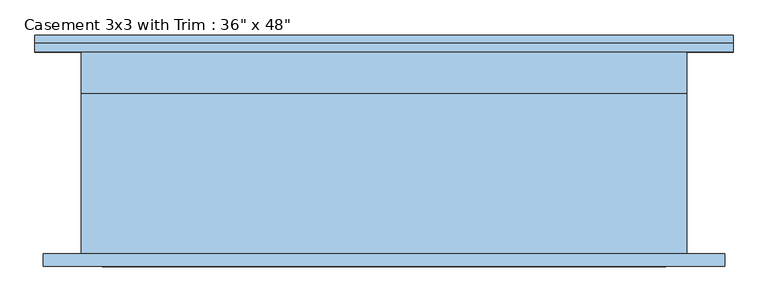
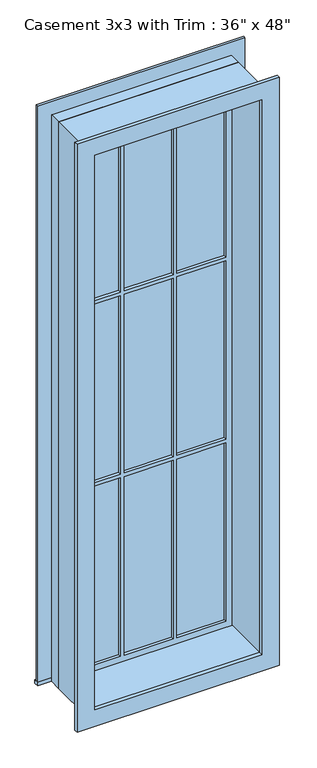
"""IFC4 building model written with IfcOpenShell, lengths in millimetres: window geometry."""

from ifc_helpers import new_model, si_unit, frame, origin, place, context, project, spatial, polyline, outline, extrude, source, transform, mapped, element, save


def window_19f256ab(model_context):
    return source(origin(), model_context, "Body", "SweptSolid", [
        extrude(outline(polyline([(-527.05, 177.8), (527.05, 177.8), (527.05, 152.4), (-527.05, 152.4), (-527.05, 177.8)])), frame((0.0, 0.0, 914.4), z_axis=(0.0, 0.0, 1.0), x_axis=(1.0, 0.0, 0.0)), (0.0, 0.0, 1.0), 19.05),
        extrude(outline(polyline([(3943.35, -438.15), (3943.35, 438.15), (933.45, 438.15), (933.45, 527.05), (4032.25, 527.05), (4032.25, -527.05), (933.45, -527.05), (933.45, -438.15), (3943.35, -438.15)])), frame((0.0, 152.4, 0.0), z_axis=(0.0, 1.0, 0.0), x_axis=(0.0, 0.0, 1.0)), (0.0, 0.0, 1.0), 12.7),
        extrude(outline(polyline([(143.9333333, 117.475), (393.7, 117.475), (393.7, 104.775), (143.9333333, 104.775), (143.9333333, 117.475)])), frame((0.0, 0.0, 2937.9333333), z_axis=(0.0, 0.0, 1.0), x_axis=(1.0, 0.0, 0.0)), (0.0, 0.0, 1.0), 960.9666667),
        extrude(outline(polyline([(-124.8833333, 117.475), (124.8833333, 117.475), (124.8833333, 104.775), (-124.8833333, 104.775), (-124.8833333, 117.475)])), frame((0.0, 0.0, 2937.9333333), z_axis=(0.0, 0.0, 1.0), x_axis=(1.0, 0.0, 0.0)), (0.0, 0.0, 1.0), 960.9666667),
        extrude(outline(polyline([(-393.7, 117.475), (-143.9333333, 117.475), (-143.9333333, 104.775), (-393.7, 104.775), (-393.7, 117.475)])), frame((0.0, 0.0, 2937.9333333), z_axis=(0.0, 0.0, 1.0), x_axis=(1.0, 0.0, 0.0)), (0.0, 0.0, 1.0), 960.9666667),
        extrude(outline(polyline([(-393.7, 117.475), (-143.9333333, 117.475), (-143.9333333, 104.775), (-393.7, 104.775), (-393.7, 117.475)])), frame((0.0, 0.0, 1957.9166667), z_axis=(0.0, 0.0, 1.0), x_axis=(1.0, 0.0, 0.0)), (0.0, 0.0, 1.0), 960.9666667),
        extrude(outline(polyline([(-124.8833333, 117.475), (124.8833333, 117.475), (124.8833333, 104.775), (-124.8833333, 104.775), (-124.8833333, 117.475)])), frame((0.0, 0.0, 1957.9166667), z_axis=(0.0, 0.0, 1.0), x_axis=(1.0, 0.0, 0.0)), (0.0, 0.0, 1.0), 960.9666667),
        extrude(outline(polyline([(143.9333333, 117.475), (393.7, 117.475), (393.7, 104.775), (143.9333333, 104.775), (143.9333333, 117.475)])), frame((0.0, 0.0, 1957.9166667), z_axis=(0.0, 0.0, 1.0), x_axis=(1.0, 0.0, 0.0)), (0.0, 0.0, 1.0), 960.9666667),
        extrude(outline(polyline([(143.9333333, 117.475), (393.7, 117.475), (393.7, 104.775), (143.9333333, 104.775), (143.9333333, 117.475)])), frame((0.0, 0.0, 977.9), z_axis=(0.0, 0.0, 1.0), x_axis=(1.0, 0.0, 0.0)), (0.0, 0.0, 1.0), 960.9666667),
        extrude(outline(polyline([(-124.8833333, 117.475), (124.8833333, 117.475), (124.8833333, 104.775), (-124.8833333, 104.775), (-124.8833333, 117.475)])), frame((0.0, 0.0, 977.9), z_axis=(0.0, 0.0, 1.0), x_axis=(1.0, 0.0, 0.0)), (0.0, 0.0, 1.0), 960.9666667),
        extrude(outline(polyline([(-393.7, 117.475), (-143.9333333, 117.475), (-143.9333333, 104.775), (-393.7, 104.775), (-393.7, 117.475)])), frame((0.0, 0.0, 977.9), z_axis=(0.0, 0.0, 1.0), x_axis=(1.0, 0.0, 0.0)), (0.0, 0.0, 1.0), 960.9666667),
        extrude(outline(polyline([(4019.55, 514.35), (4019.55, -514.35), (857.25, -514.35), (857.25, 514.35), (4019.55, 514.35)]), holes=[polyline([(3930.65, 425.45), (946.15, 425.45), (946.15, -425.45), (3930.65, -425.45), (3930.65, 425.45)])]), frame((0.0, -171.45, 0.0), z_axis=(0.0, 1.0, 0.0), x_axis=(0.0, 0.0, 1.0)), (0.0, 0.0, 1.0), 19.05),
        extrude(outline(polyline([(3943.35, -438.15), (933.45, -438.15), (933.45, 438.15), (3943.35, 438.15), (3943.35, -438.15)]), holes=[polyline([(3898.9, -143.9333333), (2937.9333333, -143.9333333), (2937.9333333, -393.7), (3898.9, -393.7), (3898.9, -143.9333333)]), polyline([(2918.8833333, -143.9333333), (1957.9166667, -143.9333333), (1957.9166667, -393.7), (2918.8833333, -393.7), (2918.8833333, -143.9333333)]), polyline([(1938.8666667, -143.9333333), (977.9, -143.9333333), (977.9, -393.7), (1938.8666667, -393.7), (1938.8666667, -143.9333333)]), polyline([(3898.9, 124.8833333), (2937.9333333, 124.8833333), (2937.9333333, -124.8833333), (3898.9, -124.8833333), (3898.9, 124.8833333)]), polyline([(2918.8833333, 124.8833333), (1957.9166667, 124.8833333), (1957.9166667, -124.8833333), (2918.8833333, -124.8833333), (2918.8833333, 124.8833333)]), polyline([(1938.8666667, 124.8833333), (977.9, 124.8833333), (977.9, -124.8833333), (1938.8666667, -124.8833333), (1938.8666667, 124.8833333)]), polyline([(3898.9, 393.7), (2937.9333333, 393.7), (2937.9333333, 143.9333333), (3898.9, 143.9333333), (3898.9, 393.7)]), polyline([(2918.8833333, 393.7), (1957.9166667, 393.7), (1957.9166667, 143.9333333), (2918.8833333, 143.9333333), (2918.8833333, 393.7)]), polyline([(1938.8666667, 393.7), (977.9, 393.7), (977.9, 143.9333333), (1938.8666667, 143.9333333), (1938.8666667, 393.7)])]), frame((0.0, 88.9, 0.0), z_axis=(0.0, 1.0, 0.0), x_axis=(0.0, 0.0, 1.0)), (0.0, 0.0, 1.0), 44.45),
        extrude(outline(polyline([(3962.4, -457.2), (914.4, -457.2), (914.4, 457.2), (3962.4, 457.2), (3962.4, -457.2)]), holes=[polyline([(3930.65, -425.45), (3930.65, 425.45), (946.15, 425.45), (946.15, -425.45), (3930.65, -425.45)])]), frame((0.0, -152.4, 0.0), z_axis=(0.0, 1.0, 0.0), x_axis=(0.0, 0.0, 1.0)), (0.0, 0.0, 1.0), 241.3),
        extrude(outline(polyline([(3962.4, 457.2), (3962.4, -457.2), (914.4, -457.2), (914.4, 457.2), (3962.4, 457.2)]), holes=[polyline([(3943.35, 438.15), (933.45, 438.15), (933.45, -438.15), (3943.35, -438.15), (3943.35, 438.15)])]), frame((0.0, 88.9, 0.0), z_axis=(0.0, 1.0, 0.0), x_axis=(0.0, 0.0, 1.0)), (0.0, 0.0, 1.0), 63.5),
    ])


if __name__ == "__main__":
    model = new_model("IFC4")
    model_context = context("Model", 3, world=origin())
    ifc_project = project(units=[si_unit("LENGTHUNIT", "METRE", prefix="MILLI")], contexts=[model_context])
    site = spatial("IfcSite", under=ifc_project)
    building = spatial("IfcBuilding", under=site)
    placement = place(None, origin())
    window_shape = window_19f256ab(model_context)
    element("IfcWindow", 1, ObjectType="Casement 3x3 with Trim : 36\" x 48\"", at=placement, inside=building, context=model_context, shape_type="MappedRepresentation", body=[
        mapped(window_shape, transform((0.0, 0.0, 0.0), x_axis=(1.0, 0.0, 0.0), y_axis=(0.0, 1.0, 0.0), z_axis=(0.0, 0.0, 1.0))),
    ])
    save(model, "model.ifc")

# Revit data of these elements
# Type "Casement 3x3 with Trim : 36\" x 48\""
#   Type Mark = "13"
#   Construction Type Id = "GSP4R"
#   Assembly Code = "B2020100"
#   Analytic Construction = "1/8 in Pilkington single glazing"
#   Visual Light Transmittance = 0.9
#   Solar Heat Gain Coefficient = 0.78
#   Heat Transfer Coefficient (U) = 0.6496 BTU/(h·ft²·°F)
#   Height = 10' - 0"
#   Default Sill Height = 3' - 0"
#   Trim Projection - Ext. = 0' - 0 1/2"
#   Trim Projection - Int. = 0' - 0 3/4"
#   Trim Width - Exterior = 0' - 3 1/2"
#   Trim Width - Interior = 0' - 3 1/2"
#   Width = 3' - 0"
#   Window Inset = 0' - 0 3/4"
#   Define Thermal Properties by = 1
#   Glass Pane Material = Glass
#   Sash Material = Roofing, EPDM Membrane
#   Trim Exterior Material = Roofing, EPDM Membrane
#   Trim Interior Material = Trim
#   Wall Closure = (empty or 0)
# Element 1 (IfcWindow, "Casement 3x3 with Trim : 36\" x 48\"")
#   Materials on its faces: "Roofing, EPDM Membrane", "Glass", "Trim"
# Materials
#   "Glass": class "Glass", colour RGB 0 128 192, transparency 0.75, Description = "Soda Lime Glass", Cost = 0
#   "Roofing, EPDM Membrane": class "Generic", colour RGB 127 127 127, transparency 0, Description = "EPDM roof membrane", Cost = 0
#   "Trim": class "Wood", colour RGB 224 178 126, transparency 0
